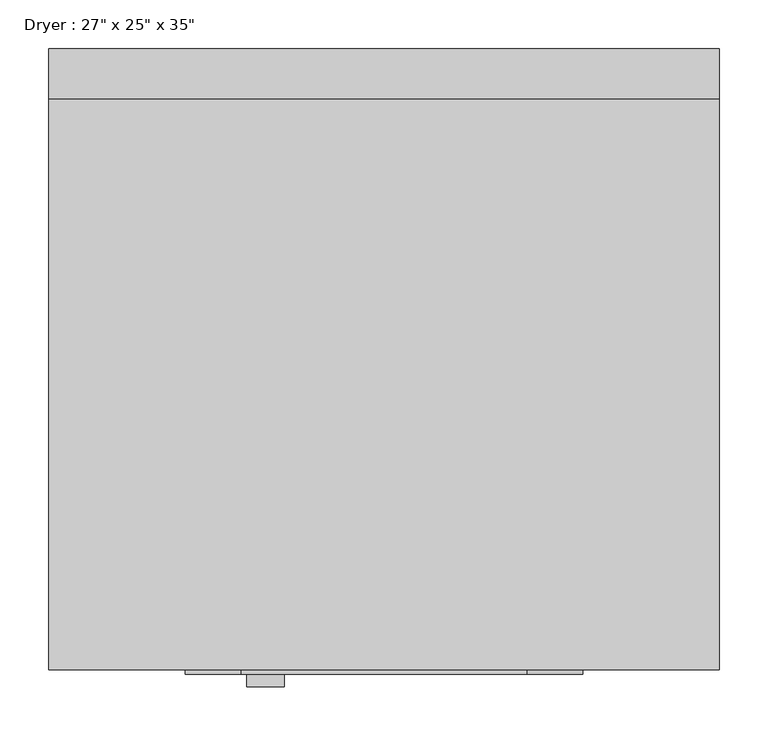
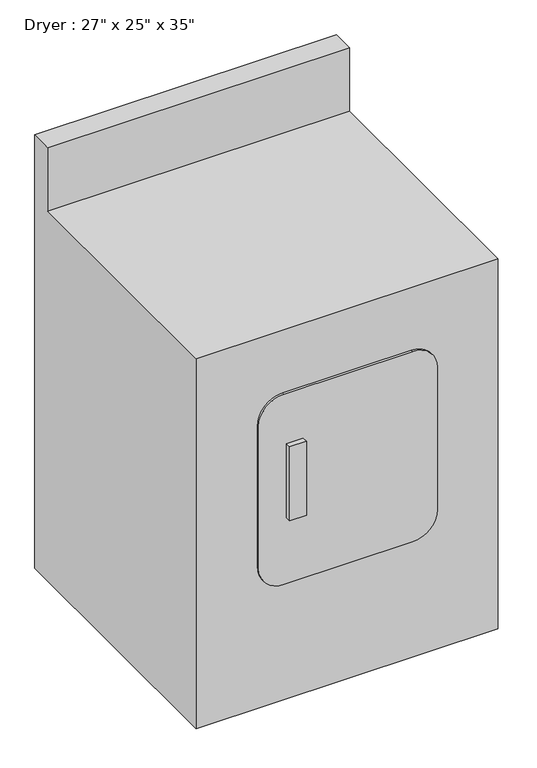
"""IFC4 building model written with IfcOpenShell, lengths in millimetres: proxy geometry."""

from ifc_helpers import new_model, si_unit, point, frame, frame_2d, origin, place, context, project, spatial, polyline, circle_curve, trimmed, segment, composite_curve, outline, extrude, source, transform, mapped, element, save


def proxy_b4d0e45e(model_context):
    return source(origin(), model_context, "Body", "SweptSolid", [
        extrude(outline(polyline([(276.7635206, -20.3014962), (238.6635206, -20.3014962), (238.6635206, -7.6014962), (276.7635206, -7.6014962), (276.7635206, -20.3014962)])), frame((0.0, 0.0, 438.7649313), z_axis=(0.0, 0.0, 1.0), x_axis=(1.0, 0.0, 0.0)), (0.0, 0.0, 1.0), 177.8),
        extrude(outline(composite_curve([segment(polyline([(737.623844, 525.0374563), (737.623844, 232.9374563)]), True, "CONTINUOUS"), segment(trimmed(circle_curve(frame_2d((680.473844, 232.9374563)), 57.15), [point((737.623844, 232.9374563))], [point((680.473844, 175.7874563))], False, "CARTESIAN"), True, "CONTINUOUS"), segment(polyline([(680.473844, 175.7874563), (337.573844, 175.7874563)]), True, "CONTINUOUS"), segment(trimmed(circle_curve(frame_2d((337.573844, 232.9374563)), 57.15), [point((337.573844, 175.7874563))], [point((280.423844, 232.9374563))], False, "CARTESIAN"), True, "CONTINUOUS"), segment(polyline([(280.423844, 232.9374563), (280.423844, 525.0374563)]), True, "CONTINUOUS"), segment(trimmed(circle_curve(frame_2d((337.573844, 525.0374563)), 57.15), [point((280.423844, 525.0374563))], [point((337.573844, 582.1874563))], False, "CARTESIAN"), True, "CONTINUOUS"), segment(polyline([(337.573844, 582.1874563), (680.473844, 582.1874563)]), True, "CONTINUOUS"), segment(trimmed(circle_curve(frame_2d((680.473844, 525.0374563)), 57.15), [point((680.473844, 582.1874563))], [point((737.623844, 525.0374563))], False, "CARTESIAN"), True, "CONTINUOUS")], self_intersect=False)), frame((0.0, -7.6014962, 0.0), z_axis=(0.0, 1.0, 0.0), x_axis=(0.0, 0.0, 1.0)), (0.0, 0.0, 1.0), 4.7625),
        extrude(outline(polyline([(632.1610038, 0.0), (-2.8389962, 0.0), (-2.8389962, 889.0), (581.3610038, 889.0), (581.3610038, 1041.4), (632.1610038, 1041.4), (632.1610038, 0.0)])), frame((36.0874563, 0.0, 0.0), z_axis=(1.0, 0.0, 0.0), x_axis=(0.0, 1.0, 0.0)), (0.0, 0.0, 1.0), 685.8),
    ])


if __name__ == "__main__":
    model = new_model("IFC4")
    model_context = context("Model", 3, world=origin())
    ifc_project = project(units=[si_unit("LENGTHUNIT", "METRE", prefix="MILLI")], contexts=[model_context])
    site = spatial("IfcSite", under=ifc_project)
    building = spatial("IfcBuilding", under=site)
    placement = place(None, origin())
    proxy_shape = proxy_b4d0e45e(model_context)
    element("IfcBuildingElementProxy", 1, Name="Dryer : 27\" x 25\" x 35\"", ObjectType="Dryer : 27\" x 25\" x 35\"", at=placement, inside=building, context=model_context, shape_type="MappedRepresentation", body=[
        mapped(proxy_shape, transform((0.0, 0.0, 0.0), x_axis=(1.0, 0.0, 0.0), y_axis=(0.0, 1.0, 0.0), z_axis=(0.0, 0.0, 1.0))),
    ])
    save(model, "model.ifc")

# Revit data of these elements
# Type "Dryer : 27\" x 25\" x 35\""
#   Label = "D"
#   Assembly Code = "E1090400"
#   Depth = 2' - 1"
#   Height = 2' - 11"
#   Width = 2' - 3"
#   Dryer Material = Steel, Paint Finish, Ivory, Glossy
#   Default Elevation = 0
# Element 1 (IfcBuildingElementProxy, "Dryer : 27\" x 25\" x 35\"")
#   Materials on its faces: "Steel, Paint Finish, Ivory, Glossy"
# Materials
#   "Steel, Paint Finish, Ivory, Glossy": class "Metal", colour RGB 247 247 239, transparency 0, Description = "Steel, paint finish, ivory, glossy", Cost = 0
